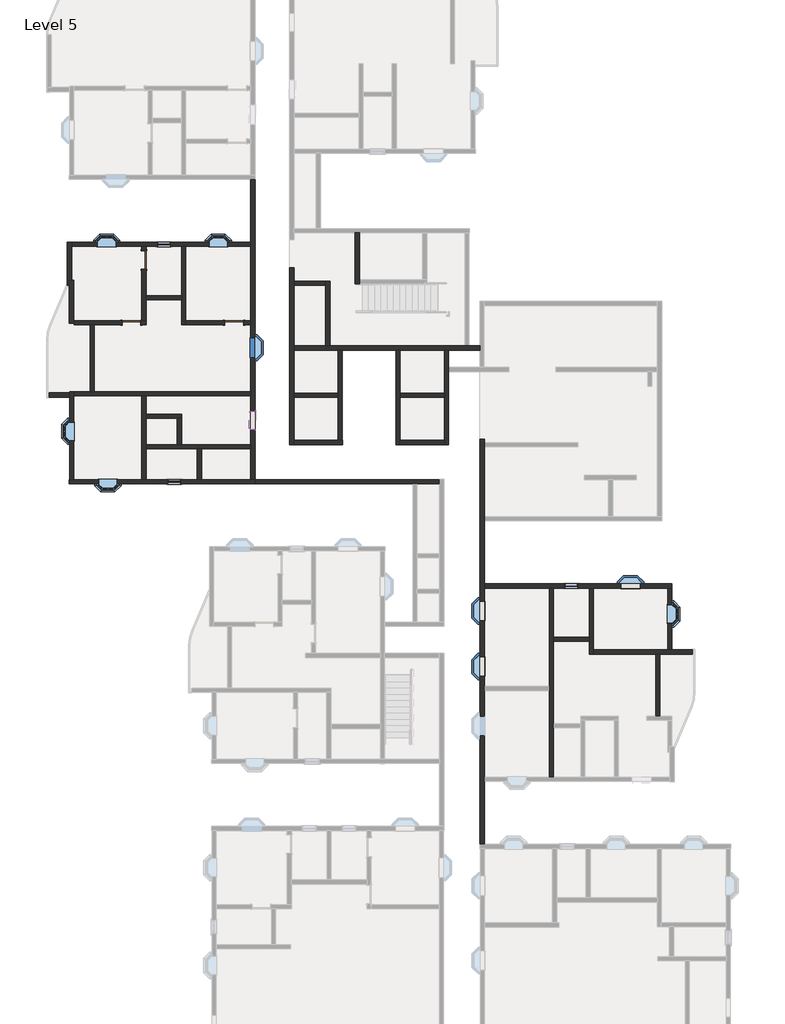
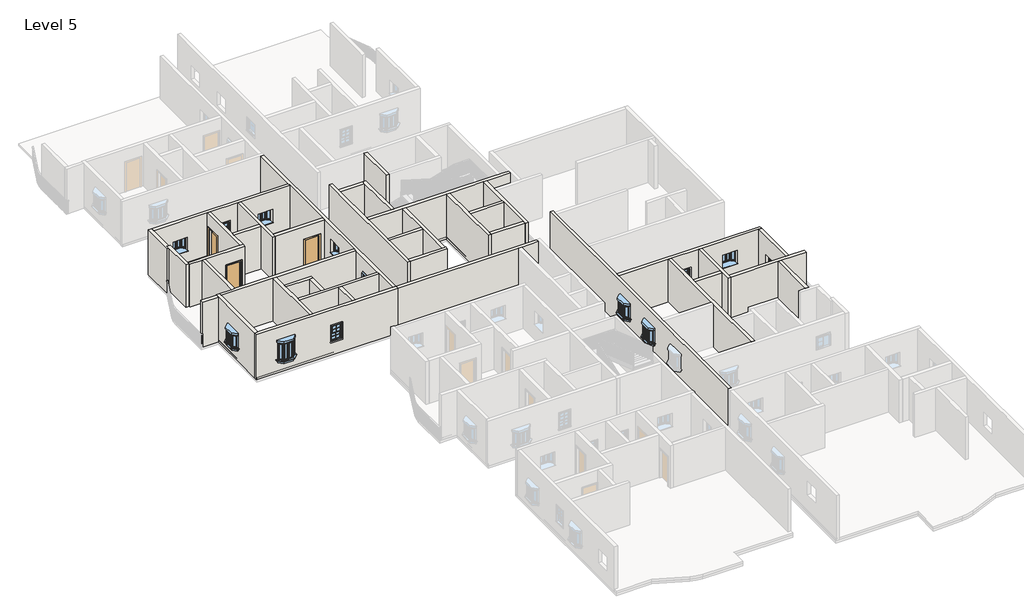
# One storey, part 3 of 14: 40 walls, 13 windows, 3 doors.
"""IFC4 building model written with IfcOpenShell, lengths in millimetres."""

from ifc_helpers import new_model, si_unit, frame, origin, place, context, project, spatial, polyline, outline, extrude, faceted_brep, transform, mapped, element, save
from components import door_54dd4da4, window_910x1210mm_154f9356, window_910x910mm_67ef725a, window_8debb0fa, windows_sgl_w_glazing_bars_910x910mm_256712d0

model = new_model("IFC4")

# Units and contexts
model_context = context("Model", 3, world=origin())
ifc_project = project(units=[si_unit("LENGTHUNIT", "METRE", prefix="MILLI")], contexts=[model_context])

# Site, building, storey
site = spatial("IfcSite", under=ifc_project)
building = spatial("IfcBuilding", under=site)
storey = spatial("IfcBuildingStorey", under=building, Name="Level 5", Elevation=12192.0)

# Doors
placement = place(None, origin())
door_shape = door_54dd4da4(model_context)
element("IfcDoor", 1, ObjectType="Single-Flush : 36\" x 84\"", at=placement, inside=storey, context=model_context, shape_type="MappedRepresentation", body=[
    mapped(door_shape, transform((-11210.3891351, 10605.7083494, 12192.0), x_axis=(1.0, 0.0, 0.0), y_axis=(0.0, 1.0, 0.0), z_axis=(0.0, 0.0, 1.0))),
])
element("IfcDoor", 2, ObjectType="Single-Flush : 36\" x 84\"", at=placement, inside=storey, context=model_context, shape_type="MappedRepresentation", body=[
    mapped(door_shape, transform((-15610.9391351, 13672.7583494, 12192.0), x_axis=(0.0, -1.0, 0.0), y_axis=(1.0, 0.0, 0.0), z_axis=(0.0, 0.0, 1.0))),
])
element("IfcDoor", 3, ObjectType="Single-Flush : 36\" x 84\"", at=placement, inside=storey, context=model_context, shape_type="MappedRepresentation", body=[
    mapped(door_shape, transform((-16220.5391351, 10605.7083494, 12192.0), x_axis=(1.0, 0.0, 0.0), y_axis=(0.0, 1.0, 0.0), z_axis=(0.0, 0.0, 1.0))),
])

# Walls
element("IfcWall", 4, ObjectType="4.5\" p", at=placement, inside=storey, context=model_context, shape_type="Brep", body=[
    faceted_brep([(-15509.3391351, 4456.3873146, 12192.0), (-13007.4391351, 4456.3873146, 12192.0), (-12804.2391351, 4456.3873146, 12192.0), (-10397.5891351, 4456.3873146, 12192.0), (-10397.5891351, 4456.3873146, 15240.0), (-12804.2391351, 4456.3873146, 15240.0), (-13007.4391351, 4456.3873146, 15240.0), (-15509.3391351, 4456.3873146, 15240.0), (-15509.3391351, 4659.5873146, 12192.0), (-15509.3391351, 4659.5873146, 15240.0), (-13985.3391351, 4659.5873146, 15240.0), (-13782.1391351, 4659.5873146, 15240.0), (-10397.5891351, 4659.5873146, 15240.0), (-10397.5891351, 4659.5873146, 12192.0), (-13782.1391351, 4659.5873146, 12192.0), (-13985.3391351, 4659.5873146, 12192.0)], [[[0, 1, 2, 3, 4, 5, 6, 7]], [[8, 9, 10, 11, 12, 13, 14, 15]], [[3, 2, 1, 0, 8, 15, 14, 13]], [[7, 6, 5, 4, 12, 11, 10, 9]], [[4, 3, 13, 12]], [[0, 7, 9, 8]]]),
])
element("IfcWall", 5, ObjectType="4.5\" p", at=placement, inside=storey, context=model_context, shape_type="SweptSolid", body=[
    extrude(outline(polyline([(-13007.4391351, 2953.9583494), (-13007.4391351, 4456.3873146), (-12804.2391351, 4456.3873146), (-12804.2391351, 2953.9583494), (-13007.4391351, 2953.9583494)])), frame((0.0, 0.0, 12192.0), z_axis=(0.0, 0.0, 1.0), x_axis=(1.0, 0.0, 0.0)), (0.0, 0.0, 1.0), 3048.0),
])
element("IfcWall", 6, ObjectType="4.5\" p", at=placement, inside=storey, context=model_context, shape_type="Brep", body=[
    faceted_brep([(-15509.3391351, 5953.2975261, 12192.0), (-13985.3391351, 5953.2975261, 12192.0), (-13782.1391351, 5953.2975261, 12192.0), (-13782.1391351, 5953.2975261, 15240.0), (-13985.3391351, 5953.2975261, 15240.0), (-15509.3391351, 5953.2975261, 15240.0), (-15509.3391351, 6156.4975261, 12192.0), (-15509.3391351, 6156.4975261, 15240.0), (-13782.1391351, 6156.4975261, 15240.0), (-13782.1391351, 6156.4975261, 12192.0)], [[[0, 1, 2, 3, 4, 5]], [[6, 7, 8, 9]], [[2, 1, 0, 6, 9]], [[5, 4, 3, 8, 7]], [[0, 5, 7, 6]], [[3, 2, 9, 8]]]),
])
element("IfcWall", 7, ObjectType="4.5\" p", at=placement, inside=storey, context=model_context, shape_type="SweptSolid", body=[
    extrude(outline(polyline([(-13985.3391351, 4659.5873146), (-13985.3391351, 5953.2975261), (-13782.1391351, 5953.2975261), (-13782.1391351, 4659.5873146), (-13985.3391351, 4659.5873146)])), frame((0.0, 0.0, 12192.0), z_axis=(0.0, 0.0, 1.0), x_axis=(1.0, 0.0, 0.0)), (0.0, 0.0, 1.0), 3048.0),
])
element("IfcWall", 8, ObjectType="4.5\" p", at=placement, inside=storey, context=model_context, shape_type="Brep", body=[
    faceted_brep([(-15712.5391351, 13215.5583494, 14325.6), (-15712.5391351, 13215.5583494, 12192.0), (-15712.5391351, 10707.3083494, 12192.0), (-15712.5391351, 10707.3083494, 15240.0), (-15712.5391351, 14333.1583494, 15240.0), (-15712.5391351, 14333.1583494, 12192.0), (-15712.5391351, 14129.9583494, 12192.0), (-15712.5391351, 14129.9583494, 14325.6), (-15509.3391351, 10707.3083494, 12192.0), (-15509.3391351, 11723.3083494, 12192.0), (-15509.3391351, 11926.5083494, 12192.0), (-15509.3391351, 13215.5583494, 12192.0), (-15509.3391351, 13215.5583494, 14325.6), (-15509.3391351, 14129.9583494, 14325.6), (-15509.3391351, 14129.9583494, 12192.0), (-15509.3391351, 14333.1583494, 12192.0), (-15509.3391351, 14333.1583494, 15240.0), (-15509.3391351, 11926.5083494, 15240.0), (-15509.3391351, 11723.3083494, 15240.0), (-15509.3391351, 10707.3083494, 15240.0)], [[[0, 1, 2, 3, 4, 5, 6, 7]], [[8, 9, 10, 11, 12, 13, 14, 15, 16, 17, 18, 19]], [[6, 5, 15, 14]], [[2, 1, 11, 10, 9, 8]], [[4, 3, 19, 18, 17, 16]], [[3, 2, 8, 19]], [[5, 4, 16, 15]], [[12, 11, 1, 0]], [[13, 12, 0, 7]], [[14, 13, 7, 6]]]),
])
element("IfcWall", 9, ObjectType="4.5\" p", at=placement, inside=storey, context=model_context, shape_type="Brep", body=[
    faceted_brep([(-13769.4391351, 14333.1583494, 12192.0), (-13769.4391351, 11926.5083494, 12192.0), (-13769.4391351, 11723.3083494, 12192.0), (-13769.4391351, 10504.1083494, 12192.0), (-13769.4391351, 10504.1083494, 15240.0), (-13769.4391351, 11723.3083494, 15240.0), (-13769.4391351, 11926.5083494, 15240.0), (-13769.4391351, 14333.1583494, 15240.0), (-13566.2391351, 14333.1583494, 12192.0), (-13566.2391351, 14333.1583494, 15240.0), (-13566.2391351, 10707.3083494, 15240.0), (-13566.2391351, 10504.1083494, 15240.0), (-13566.2391351, 10504.1083494, 12192.0), (-13566.2391351, 10707.3083494, 12192.0)], [[[0, 1, 2, 3, 4, 5, 6, 7]], [[8, 9, 10, 11, 12, 13]], [[3, 2, 1, 0, 8, 13, 12]], [[7, 6, 5, 4, 11, 10, 9]], [[0, 7, 9, 8]], [[4, 3, 12, 11]]]),
])
element("IfcWall", 10, ObjectType="4.5\" p", at=placement, inside=storey, context=model_context, shape_type="SweptSolid", body=[
    extrude(outline(polyline([(14325.6, -10753.1891351), (12192.0, -10753.1891351), (12192.0, -10397.5891351), (15240.0, -10397.5891351), (15240.0, -13566.2391351), (12192.0, -13566.2391351), (12192.0, -11667.5891351), (14325.6, -11667.5891351), (14325.6, -10753.1891351)])), frame((0.0, 10504.1083494, 0.0), z_axis=(0.0, 1.0, 0.0), x_axis=(0.0, 0.0, 1.0)), (0.0, 0.0, 1.0), 203.2),
])
element("IfcWall", 11, ObjectType="4.5\" p", at=placement, inside=storey, context=model_context, shape_type="SweptSolid", body=[
    extrude(outline(polyline([(-13769.4391351, 11723.3083494), (-15509.3391351, 11723.3083494), (-15509.3391351, 11926.5083494), (-13769.4391351, 11926.5083494), (-13769.4391351, 11723.3083494)])), frame((0.0, 0.0, 12192.0), z_axis=(0.0, 0.0, 1.0), x_axis=(1.0, 0.0, 0.0)), (0.0, 0.0, 1.0), 3048.0),
])
element("IfcWall", 12, ObjectType="4.5\" p", at=placement, inside=storey, context=model_context, shape_type="SweptSolid", body=[
    extrude(outline(polyline([(-6739.9891351, 12429.8715905), (-8289.3891351, 12429.8715905), (-8289.3891351, 12633.0715905), (-6739.9891351, 12633.0715905), (-6739.9891351, 12429.8715905)])), frame((0.0, 0.0, 12192.0), z_axis=(0.0, 0.0, 1.0), x_axis=(1.0, 0.0, 0.0)), (0.0, 0.0, 1.0), 3048.0),
])
element("IfcWall", 13, ObjectType="4.5\" p", at=placement, inside=storey, context=model_context, shape_type="SweptSolid", body=[
    extrude(outline(polyline([(-6130.3891351, 6970.2449943), (-8289.3891351, 6970.2449943), (-8289.3891351, 7173.4449943), (-6130.3891351, 7173.4449943), (-6130.3891351, 6970.2449943)])), frame((0.0, 0.0, 12192.0), z_axis=(0.0, 0.0, 1.0), x_axis=(1.0, 0.0, 0.0)), (0.0, 0.0, 1.0), 3048.0),
])
element("IfcWall", 14, ObjectType="4.5\" p", at=placement, inside=storey, context=model_context, shape_type="SweptSolid", body=[
    extrude(outline(polyline([(-948.7891351, 6970.2449943), (-3107.7891351, 6970.2449943), (-3107.7891351, 7173.4449943), (-948.7891351, 7173.4449943), (-948.7891351, 6970.2449943)])), frame((0.0, 0.0, 12192.0), z_axis=(0.0, 0.0, 1.0), x_axis=(1.0, 0.0, 0.0)), (0.0, 0.0, 1.0), 3048.0),
])
element("IfcWall", 15, ObjectType="4.5\" p", at=placement, inside=storey, context=model_context, shape_type="Brep", body=[
    faceted_brep([(-5298.5391351, 14988.9215905, 12192.0), (-5298.5391351, 12506.0715905, 12192.0), (-5298.5391351, 12506.0715905, 15240.0), (-5298.5391351, 14988.9215905, 15240.0), (-5095.3391351, 14988.9215905, 12192.0), (-5095.3391351, 14988.9215905, 15240.0), (-5095.3391351, 12709.2715905, 15240.0), (-5095.3391351, 12506.0715905, 15240.0), (-5095.3391351, 12506.0715905, 12192.0), (-5095.3391351, 12709.2715905, 12192.0)], [[[0, 1, 2, 3]], [[4, 5, 6, 7, 8, 9]], [[1, 0, 4, 9, 8]], [[3, 2, 7, 6, 5]], [[0, 3, 5, 4]], [[2, 1, 8, 7]]]),
])
element("IfcWall", 16, ObjectType="4.5\" p", at=placement, inside=storey, context=model_context, shape_type="SweptSolid", body=[
    extrude(outline(polyline([(-948.7891351, 4665.1949943), (-3107.7891351, 4665.1949943), (-3107.7891351, 4868.3949943), (-948.7891351, 4868.3949943), (-948.7891351, 4665.1949943)])), frame((0.0, 0.0, 12192.0), z_axis=(0.0, 0.0, 1.0), x_axis=(1.0, 0.0, 0.0)), (0.0, 0.0, 1.0), 3048.0),
])
element("IfcWall", 17, ObjectType="4.5\" p", at=placement, inside=storey, context=model_context, shape_type="Brep", body=[
    faceted_brep([(4184.4880523, -2336.4042694, 12192.0), (4184.4880523, -7130.6542694, 12192.0), (4184.4880523, -7333.8542694, 12192.0), (4184.4880523, -11556.6042694, 12192.0), (4184.4880523, -11556.6042694, 15240.0), (4184.4880523, -7333.8542694, 15240.0), (4184.4880523, -7130.6542694, 15240.0), (4184.4880523, -2336.4042694, 15240.0), (4387.6880523, -2336.4042694, 12192.0), (4387.6880523, -2336.4042694, 15240.0), (4387.6880523, -4736.7042694, 15240.0), (4387.6880523, -4939.9042694, 15240.0), (4387.6880523, -8959.4542694, 15240.0), (4387.6880523, -9162.6542694, 15240.0), (4387.6880523, -11556.6042694, 15240.0), (4387.6880523, -11556.6042694, 12192.0), (4387.6880523, -9162.6542694, 12192.0), (4387.6880523, -8959.4542694, 12192.0), (4387.6880523, -4939.9042694, 12192.0), (4387.6880523, -4736.7042694, 12192.0)], [[[0, 1, 2, 3, 4, 5, 6, 7]], [[8, 9, 10, 11, 12, 13, 14, 15, 16, 17, 18, 19]], [[3, 2, 1, 0, 8, 19, 18, 17, 16, 15]], [[7, 6, 5, 4, 14, 13, 12, 11, 10, 9]], [[4, 3, 15, 14]], [[0, 7, 9, 8]]]),
])
element("IfcWall", 18, ObjectType="4.5\" p", at=placement, inside=storey, context=model_context, shape_type="Brep", body=[
    faceted_brep([(803.8108649, 4915.2957306, 12192.0), (803.8108649, -14845.9042694, 12192.0), (803.8108649, -14845.9042694, 15240.0), (803.8108649, 4915.2957306, 15240.0), (803.8108649, -9516.0542694, 14302.0), (803.8108649, -9516.0542694, 13392.0), (803.8108649, -8606.0542694, 13392.0), (803.8108649, -8606.0542694, 14302.0), (803.8108649, -3909.0042694, 14302.0), (803.8108649, -3909.0042694, 13392.0), (803.8108649, -2999.0042694, 13392.0), (803.8108649, -2999.0042694, 14302.0), (803.8108649, -6620.4542694, 14302.0), (803.8108649, -6620.4542694, 13392.0), (803.8108649, -5710.4542694, 13392.0), (803.8108649, -5710.4542694, 14302.0), (1007.0108649, 4915.2957306, 12192.0), (1007.0108649, 4915.2957306, 15240.0), (1007.0108649, 4754.0949943, 15240.0), (1007.0108649, 4550.8949943, 15240.0), (1007.0108649, 1143.3957306, 15240.0), (1007.0108649, 940.1957306, 15240.0), (1007.0108649, -2133.2042694, 15240.0), (1007.0108649, -2336.4042694, 15240.0), (1007.0108649, -7130.6542694, 15240.0), (1007.0108649, -7333.8542694, 15240.0), (1007.0108649, -11556.6042694, 15240.0), (1007.0108649, -11759.8042694, 15240.0), (1007.0108649, -14845.9042694, 15240.0), (1007.0108649, -14845.9042694, 12192.0), (1007.0108649, -11759.8042694, 12192.0), (1007.0108649, -11556.6042694, 12192.0), (1007.0108649, -7333.8542694, 12192.0), (1007.0108649, -7130.6542694, 12192.0), (1007.0108649, -2336.4042694, 12192.0), (1007.0108649, -2133.2042694, 12192.0), (1007.0108649, 940.1957306, 12192.0), (1007.0108649, 1143.3957306, 12192.0), (1007.0108649, 4550.8949943, 12192.0), (1007.0108649, 4754.0949943, 12192.0), (1007.0108649, -9516.0542694, 14302.0), (1007.0108649, -8606.0542694, 14302.0), (1007.0108649, -8606.0542694, 13392.0), (1007.0108649, -9516.0542694, 13392.0), (1007.0108649, -3909.0042694, 14302.0), (1007.0108649, -2999.0042694, 14302.0), (1007.0108649, -2999.0042694, 13392.0), (1007.0108649, -3909.0042694, 13392.0), (1007.0108649, -6620.4542694, 14302.0), (1007.0108649, -5710.4542694, 14302.0), (1007.0108649, -5710.4542694, 13392.0), (1007.0108649, -6620.4542694, 13392.0)], [[[0, 1, 2, 3], [4, 5, 6, 7], [8, 9, 10, 11], [12, 13, 14, 15]], [[16, 17, 18, 19, 20, 21, 22, 23, 24, 25, 26, 27, 28, 29, 30, 31, 32, 33, 34, 35, 36, 37, 38, 39], [40, 41, 42, 43], [44, 45, 46, 47], [48, 49, 50, 51]], [[1, 0, 16, 39, 38, 37, 36, 35, 34, 33, 32, 31, 30, 29]], [[3, 2, 28, 27, 26, 25, 24, 23, 22, 21, 20, 19, 18, 17]], [[0, 3, 17, 16]], [[2, 1, 29, 28]], [[5, 4, 40, 43]], [[6, 5, 43, 42]], [[7, 6, 42, 41]], [[4, 7, 41, 40]], [[9, 8, 44, 47]], [[10, 9, 47, 46]], [[11, 10, 46, 45]], [[8, 11, 45, 44]], [[13, 12, 48, 51]], [[14, 13, 51, 50]], [[15, 14, 50, 49]], [[12, 15, 49, 48]]]),
])
element("IfcWall", 19, ObjectType="4.5\" p", at=placement, inside=storey, context=model_context, shape_type="SweptSolid", body=[
    extrude(outline(polyline([(6127.5880523, -4939.9042694), (4387.6880523, -4939.9042694), (4387.6880523, -4736.7042694), (6127.5880523, -4736.7042694), (6127.5880523, -4939.9042694)])), frame((0.0, 0.0, 12192.0), z_axis=(0.0, 0.0, 1.0), x_axis=(1.0, 0.0, 0.0)), (0.0, 0.0, 1.0), 3048.0),
])
element("IfcWall", 20, ObjectType="4.5\" p", at=placement, inside=storey, context=model_context, shape_type="Brep", body=[
    faceted_brep([(6127.5880523, -2336.4042694, 12192.0), (6127.5880523, -4736.7042694, 12192.0), (6127.5880523, -4939.9042694, 12192.0), (6127.5880523, -5555.8542694, 12192.0), (6127.5880523, -5555.8542694, 15240.0), (6127.5880523, -4939.9042694, 15240.0), (6127.5880523, -4736.7042694, 15240.0), (6127.5880523, -2336.4042694, 15240.0), (6330.7880523, -2336.4042694, 12192.0), (6330.7880523, -2336.4042694, 15240.0), (6330.7880523, -5352.6542694, 15240.0), (6330.7880523, -5555.8542694, 15240.0), (6330.7880523, -5555.8542694, 12192.0), (6330.7880523, -5352.6542694, 12192.0)], [[[0, 1, 2, 3, 4, 5, 6, 7]], [[8, 9, 10, 11, 12, 13]], [[3, 2, 1, 0, 8, 13, 12]], [[7, 6, 5, 4, 11, 10, 9]], [[0, 7, 9, 8]], [[4, 3, 12, 11]]]),
])
element("IfcWall", 21, ObjectType="4.5\" p", at=placement, inside=storey, context=model_context, shape_type="Brep", body=[
    faceted_brep([(6330.7880523, -5555.8542694, 12192.0), (9371.2322031, -5555.8542694, 12192.0), (9574.4322031, -5555.8542694, 12192.0), (11163.1380523, -5555.8542694, 12192.0), (11163.1380523, -5555.8542694, 15240.0), (9574.4322031, -5555.8542694, 15240.0), (9371.2322031, -5555.8542694, 15240.0), (6330.7880523, -5555.8542694, 15240.0), (6330.7880523, -5352.6542694, 12192.0), (6330.7880523, -5352.6542694, 15240.0), (9956.6380523, -5352.6542694, 15240.0), (10159.8380523, -5352.6542694, 15240.0), (11163.1380523, -5352.6542694, 15240.0), (11163.1380523, -5352.6542694, 12192.0), (10159.8380523, -5352.6542694, 12192.0), (9956.6380523, -5352.6542694, 12192.0)], [[[0, 1, 2, 3, 4, 5, 6, 7]], [[8, 9, 10, 11, 12, 13, 14, 15]], [[3, 2, 1, 0, 8, 15, 14, 13]], [[4, 3, 13, 12]], [[7, 6, 5, 4, 12, 11, 10, 9]], [[0, 7, 9, 8]]]),
])
element("IfcWall", 22, ObjectType="4.5\" p", at=placement, inside=storey, context=model_context, shape_type="SweptSolid", body=[
    extrude(outline(polyline([(9371.2322031, -8578.4542694), (9371.2322031, -5555.8542694), (9574.4322031, -5555.8542694), (9574.4322031, -8578.4542694), (9371.2322031, -8578.4542694)])), frame((0.0, 0.0, 12192.0), z_axis=(0.0, 0.0, 1.0), x_axis=(1.0, 0.0, 0.0)), (0.0, 0.0, 1.0), 3048.0),
])
element("IfcWall", 23, ObjectType="9\"", at=placement, inside=storey, context=model_context, shape_type="Brep", body=[
    faceted_brep([(-10181.6891351, 2953.9583494, 12192.0), (-10194.3891351, 2953.9583494, 12192.0), (-10397.5891351, 2953.9583494, 12192.0), (-12804.2391351, 2953.9583494, 12192.0), (-13007.4391351, 2953.9583494, 12192.0), (-15509.3391351, 2953.9583494, 12192.0), (-15712.5391351, 2953.9583494, 12192.0), (-19033.5891351, 2953.9583494, 12192.0), (-19236.7891351, 2953.9583494, 12192.0), (-19249.4891351, 2953.9583494, 12192.0), (-19249.4891351, 2953.9583494, 15240.0), (-19236.7891351, 2953.9583494, 15240.0), (-19033.5891351, 2953.9583494, 15240.0), (-15712.5391351, 2953.9583494, 15240.0), (-15509.3391351, 2953.9583494, 15240.0), (-13007.4391351, 2953.9583494, 15240.0), (-12804.2391351, 2953.9583494, 15240.0), (-10397.5891351, 2953.9583494, 15240.0), (-10194.3891351, 2953.9583494, 15240.0), (-10181.6891351, 2953.9583494, 15240.0), (-13794.8391351, 2953.9583494, 14173.2), (-14455.2391351, 2953.9583494, 14173.2), (-14455.2391351, 2953.9583494, 13106.4), (-13794.8391351, 2953.9583494, 13106.4), (-16918.0641351, 2953.9583494, 14302.0), (-17828.0641351, 2953.9583494, 14302.0), (-17828.0641351, 2953.9583494, 13092.0), (-16918.0641351, 2953.9583494, 13092.0), (-10181.6891351, 2750.7583494, 12192.0), (-10181.6891351, 2750.7583494, 15240.0), (-19249.4891351, 2750.7583494, 15240.0), (-19249.4891351, 2750.7583494, 12192.0), (-13794.8391351, 2750.7583494, 14173.2), (-13794.8391351, 2750.7583494, 13106.4), (-14455.2391351, 2750.7583494, 13106.4), (-14455.2391351, 2750.7583494, 14173.2), (-16918.0641351, 2750.7583494, 14302.0), (-16918.0641351, 2750.7583494, 13092.0), (-17828.0641351, 2750.7583494, 13092.0), (-17828.0641351, 2750.7583494, 14302.0)], [[[0, 1, 2, 3, 4, 5, 6, 7, 8, 9, 10, 11, 12, 13, 14, 15, 16, 17, 18, 19], [20, 21, 22, 23], [24, 25, 26, 27]], [[28, 29, 30, 31], [32, 33, 34, 35], [36, 37, 38, 39]], [[9, 8, 7, 6, 5, 4, 3, 2, 1, 0, 28, 31]], [[10, 9, 31, 30]], [[19, 18, 17, 16, 15, 14, 13, 12, 11, 10, 30, 29]], [[0, 19, 29, 28]], [[33, 32, 20, 23]], [[34, 33, 23, 22]], [[35, 34, 22, 21]], [[32, 35, 21, 20]], [[37, 36, 24, 27]], [[38, 37, 27, 26]], [[39, 38, 26, 25]], [[36, 39, 25, 24]]]),
])
element("IfcWall", 24, ObjectType="9\"", at=placement, inside=storey, context=model_context, shape_type="Brep", body=[
    faceted_brep([(-19033.5891351, 2953.9583494, 12192.0), (-19033.5891351, 7037.0083494, 12192.0), (-19033.5891351, 7240.2083494, 12192.0), (-19033.5891351, 7240.2083494, 15240.0), (-19033.5891351, 7037.0083494, 15240.0), (-19033.5891351, 2953.9583494, 15240.0), (-19033.5891351, 4854.8083494, 14016.4), (-19033.5891351, 5764.8083494, 14016.4), (-19033.5891351, 5764.8083494, 13106.4), (-19033.5891351, 4854.8083494, 13106.4), (-19236.7891351, 2953.9583494, 12192.0), (-19236.7891351, 2953.9583494, 15240.0), (-19236.7891351, 7240.2083494, 15240.0), (-19236.7891351, 7240.2083494, 12192.0), (-19236.7891351, 4854.8083494, 14016.4), (-19236.7891351, 4854.8083494, 13106.4), (-19236.7891351, 5764.8083494, 13106.4), (-19236.7891351, 5764.8083494, 14016.4)], [[[0, 1, 2, 3, 4, 5], [6, 7, 8, 9]], [[10, 11, 12, 13], [14, 15, 16, 17]], [[2, 1, 0, 10, 13]], [[5, 4, 3, 12, 11]], [[0, 5, 11, 10]], [[3, 2, 13, 12]], [[15, 14, 6, 9]], [[16, 15, 9, 8]], [[17, 16, 8, 7]], [[14, 17, 7, 6]]]),
])
element("IfcWall", 25, ObjectType="9\"", at=placement, inside=storey, context=model_context, shape_type="Brep", body=[
    faceted_brep([(-10194.3891351, 2953.9583494, 12192.0), (-10194.3891351, 17597.0583494, 12192.0), (-10194.3891351, 17597.0583494, 15240.0), (-10194.3891351, 2953.9583494, 15240.0), (-10194.3891351, 9841.5083494, 14302.0), (-10194.3891351, 9841.5083494, 13392.0), (-10194.3891351, 8931.5083494, 13392.0), (-10194.3891351, 8931.5083494, 14302.0), (-10194.3891351, 5393.297832, 14302.0), (-10194.3891351, 6303.297832, 14302.0), (-10194.3891351, 6303.297832, 13392.0), (-10194.3891351, 5393.297832, 13392.0), (-10397.5891351, 2953.9583494, 12192.0), (-10397.5891351, 2953.9583494, 15240.0), (-10397.5891351, 4456.3873146, 15240.0), (-10397.5891351, 4659.5873146, 15240.0), (-10397.5891351, 7037.0083494, 15240.0), (-10397.5891351, 7240.2083494, 15240.0), (-10397.5891351, 10504.1083494, 15240.0), (-10397.5891351, 10707.3083494, 15240.0), (-10397.5891351, 14333.1583494, 15240.0), (-10397.5891351, 14536.3583494, 15240.0), (-10397.5891351, 17597.0583494, 15240.0), (-10397.5891351, 17597.0583494, 12192.0), (-10397.5891351, 14536.3583494, 12192.0), (-10397.5891351, 14333.1583494, 12192.0), (-10397.5891351, 10707.3083494, 12192.0), (-10397.5891351, 10504.1083494, 12192.0), (-10397.5891351, 7240.2083494, 12192.0), (-10397.5891351, 7037.0083494, 12192.0), (-10397.5891351, 4659.5873146, 12192.0), (-10397.5891351, 4456.3873146, 12192.0), (-10397.5891351, 9841.5083494, 14302.0), (-10397.5891351, 8931.5083494, 14302.0), (-10397.5891351, 8931.5083494, 13392.0), (-10397.5891351, 9841.5083494, 13392.0), (-10397.5891351, 5393.297832, 14302.0), (-10397.5891351, 5393.297832, 13392.0), (-10397.5891351, 6303.297832, 13392.0), (-10397.5891351, 6303.297832, 14302.0)], [[[0, 1, 2, 3], [4, 5, 6, 7], [8, 9, 10, 11]], [[12, 13, 14, 15, 16, 17, 18, 19, 20, 21, 22, 23, 24, 25, 26, 27, 28, 29, 30, 31], [32, 33, 34, 35], [36, 37, 38, 39]], [[1, 0, 12, 31, 30, 29, 28, 27, 26, 25, 24, 23]], [[2, 1, 23, 22]], [[3, 2, 22, 21, 20, 19, 18, 17, 16, 15, 14, 13]], [[0, 3, 13, 12]], [[5, 4, 32, 35]], [[6, 5, 35, 34]], [[7, 6, 34, 33]], [[4, 7, 33, 32]], [[37, 36, 8, 11]], [[38, 37, 11, 10]], [[39, 38, 10, 9]], [[36, 39, 9, 8]]]),
])
element("IfcWall", 26, ObjectType="9\"", at=placement, inside=storey, context=model_context, shape_type="SweptSolid", body=[
    extrude(outline(polyline([(-19249.4891351, 6979.8583494), (-20240.0891351, 6979.8583494), (-20240.0891351, 7183.0583494), (-19249.4891351, 7183.0583494), (-19249.4891351, 6979.8583494)])), frame((0.0, 0.0, 12192.0), z_axis=(0.0, 0.0, 1.0), x_axis=(1.0, 0.0, 0.0)), (0.0, 0.0, 1.0), 3048.0),
])
element("IfcWall", 27, ObjectType="9\"", at=placement, inside=storey, context=model_context, shape_type="Brep", body=[
    faceted_brep([(-19147.8891351, 12435.1858981, 12192.0), (-19147.8891351, 14333.1583494, 12192.0), (-19147.8891351, 14536.3583494, 12192.0), (-19147.8891351, 14549.0583494, 12192.0), (-19147.8891351, 14549.0583494, 15240.0), (-19147.8891351, 14536.3583494, 15240.0), (-19147.8891351, 14333.1583494, 15240.0), (-19147.8891351, 12435.1858981, 15240.0), (-19351.0891351, 12435.1858981, 12192.0), (-19351.0891351, 12435.1858981, 15240.0), (-19351.0891351, 14549.0583494, 15240.0), (-19351.0891351, 14549.0583494, 12192.0)], [[[0, 1, 2, 3, 4, 5, 6, 7]], [[8, 9, 10, 11]], [[3, 2, 1, 0, 8, 11]], [[4, 3, 11, 10]], [[7, 6, 5, 4, 10, 9]], [[0, 7, 9, 8]]]),
])
element("IfcWall", 28, ObjectType="9\"", at=placement, inside=storey, context=model_context, shape_type="Brep", body=[
    faceted_brep([(-19147.8891351, 14333.1583494, 12192.0), (-15712.5391351, 14333.1583494, 12192.0), (-15509.3391351, 14333.1583494, 12192.0), (-13769.4391351, 14333.1583494, 12192.0), (-13566.2391351, 14333.1583494, 12192.0), (-10397.5891351, 14333.1583494, 12192.0), (-10397.5891351, 14333.1583494, 15240.0), (-13566.2391351, 14333.1583494, 15240.0), (-13769.4391351, 14333.1583494, 15240.0), (-15509.3391351, 14333.1583494, 15240.0), (-15712.5391351, 14333.1583494, 15240.0), (-19147.8891351, 14333.1583494, 15240.0), (-17885.2141351, 14333.1583494, 14016.4), (-16975.2141351, 14333.1583494, 14016.4), (-16975.2141351, 14333.1583494, 13106.4), (-17885.2141351, 14333.1583494, 13106.4), (-12436.9141351, 14333.1583494, 14016.4), (-11526.9141351, 14333.1583494, 14016.4), (-11526.9141351, 14333.1583494, 13106.4), (-12436.9141351, 14333.1583494, 13106.4), (-14309.1891351, 14333.1583494, 14173.2), (-14309.1891351, 14333.1583494, 13106.4), (-14969.5891351, 14333.1583494, 13106.4), (-14969.5891351, 14333.1583494, 14173.2), (-19147.8891351, 14536.3583494, 12192.0), (-19147.8891351, 14536.3583494, 15240.0), (-10397.5891351, 14536.3583494, 15240.0), (-10397.5891351, 14536.3583494, 12192.0), (-17885.2141351, 14536.3583494, 14016.4), (-17885.2141351, 14536.3583494, 13106.4), (-16975.2141351, 14536.3583494, 13106.4), (-16975.2141351, 14536.3583494, 14016.4), (-12436.9141351, 14536.3583494, 14016.4), (-12436.9141351, 14536.3583494, 13106.4), (-11526.9141351, 14536.3583494, 13106.4), (-11526.9141351, 14536.3583494, 14016.4), (-14309.1891351, 14536.3583494, 14173.2), (-14969.5891351, 14536.3583494, 14173.2), (-14969.5891351, 14536.3583494, 13106.4), (-14309.1891351, 14536.3583494, 13106.4)], [[[0, 1, 2, 3, 4, 5, 6, 7, 8, 9, 10, 11], [12, 13, 14, 15], [16, 17, 18, 19], [20, 21, 22, 23]], [[24, 25, 26, 27], [28, 29, 30, 31], [32, 33, 34, 35], [36, 37, 38, 39]], [[5, 4, 3, 2, 1, 0, 24, 27]], [[11, 10, 9, 8, 7, 6, 26, 25]], [[6, 5, 27, 26]], [[0, 11, 25, 24]], [[29, 28, 12, 15]], [[30, 29, 15, 14]], [[31, 30, 14, 13]], [[28, 31, 13, 12]], [[33, 32, 16, 19]], [[34, 33, 19, 18]], [[35, 34, 18, 17]], [[32, 35, 17, 16]], [[21, 20, 36, 39]], [[22, 21, 39, 38]], [[23, 22, 38, 37]], [[20, 23, 37, 36]]]),
])
element("IfcWall", 29, ObjectType="9\"", at=placement, inside=storey, context=model_context, shape_type="SweptSolid", body=[
    extrude(outline(polyline([(-19249.4891351, 10585.5474528), (-19249.4891351, 12672.4473407), (-19046.2891351, 12672.4473407), (-19046.2891351, 10585.5474528), (-19249.4891351, 10585.5474528)])), frame((0.0, 0.0, 12192.0), z_axis=(0.0, 0.0, 1.0), x_axis=(1.0, 0.0, 0.0)), (0.0, 0.0, 1.0), 3048.0),
])
element("IfcWall", 30, ObjectType="9\" w", at=placement, inside=storey, context=model_context, shape_type="Brep", body=[
    faceted_brep([(-1177.3891351, 2953.9583494, 12192.0), (-10181.6891351, 2953.9583494, 12192.0), (-10181.6891351, 2953.9583494, 15240.0), (-1177.3891351, 2953.9583494, 15240.0), (-1177.3891351, 2750.7583494, 12192.0), (-1177.3891351, 2750.7583494, 15240.0), (-2269.5891351, 2750.7583494, 15240.0), (-2472.7891351, 2750.7583494, 15240.0), (-10181.6891351, 2750.7583494, 15240.0), (-10181.6891351, 2750.7583494, 12192.0), (-2472.7891351, 2750.7583494, 12192.0), (-2269.5891351, 2750.7583494, 12192.0)], [[[0, 1, 2, 3]], [[4, 5, 6, 7, 8, 9, 10, 11]], [[1, 0, 4, 11, 10, 9]], [[2, 1, 9, 8]], [[3, 2, 8, 7, 6, 5]], [[0, 3, 5, 4]]]),
])
element("IfcWall", 31, ObjectType="9\" w", at=placement, inside=storey, context=model_context, shape_type="Brep", body=[
    faceted_brep([(-15763.3391351, 10504.1083494, 14325.6), (-15763.3391351, 10504.1083494, 12192.0), (-15509.3391351, 10504.1083494, 12192.0), (-15509.3391351, 10504.1083494, 15240.0), (-18042.9891351, 10504.1083494, 15240.0), (-18246.1891351, 10504.1083494, 15240.0), (-19027.2391351, 10504.1083494, 15240.0), (-19027.2391351, 10504.1083494, 12192.0), (-18246.1891351, 10504.1083494, 12192.0), (-18042.9891351, 10504.1083494, 12192.0), (-16677.7391351, 10504.1083494, 12192.0), (-16677.7391351, 10504.1083494, 14325.6), (-15509.3391351, 10707.3083494, 12192.0), (-15712.5391351, 10707.3083494, 12192.0), (-15763.3391351, 10707.3083494, 12192.0), (-15763.3391351, 10707.3083494, 14325.6), (-16677.7391351, 10707.3083494, 14325.6), (-16677.7391351, 10707.3083494, 12192.0), (-19027.2391351, 10707.3083494, 12192.0), (-19027.2391351, 10707.3083494, 15240.0), (-15712.5391351, 10707.3083494, 15240.0), (-15509.3391351, 10707.3083494, 15240.0)], [[[0, 1, 2, 3, 4, 5, 6, 7, 8, 9, 10, 11]], [[12, 13, 14, 15, 16, 17, 18, 19, 20, 21]], [[2, 1, 14, 13, 12]], [[10, 9, 8, 7, 18, 17]], [[6, 5, 4, 3, 21, 20, 19]], [[7, 6, 19, 18]], [[3, 2, 12, 21]], [[15, 14, 1, 0]], [[16, 15, 0, 11]], [[17, 16, 11, 10]]]),
])
element("IfcWall", 32, ObjectType="9\" w", at=placement, inside=storey, context=model_context, shape_type="SweptSolid", body=[
    extrude(outline(polyline([(-18246.1891351, 7240.2083494), (-18246.1891351, 10504.1083494), (-18042.9891351, 10504.1083494), (-18042.9891351, 7240.2083494), (-18246.1891351, 7240.2083494)])), frame((0.0, 0.0, 12192.0), z_axis=(0.0, 0.0, 1.0), x_axis=(1.0, 0.0, 0.0)), (0.0, 0.0, 1.0), 3048.0),
])
element("IfcWall", 33, ObjectType="9\" w", at=placement, inside=storey, context=model_context, shape_type="Brep", body=[
    faceted_brep([(-19033.5891351, 7037.0083494, 12192.0), (-15712.5391351, 7037.0083494, 12192.0), (-15509.3391351, 7037.0083494, 12192.0), (-10397.5891351, 7037.0083494, 12192.0), (-10397.5891351, 7037.0083494, 15240.0), (-15509.3391351, 7037.0083494, 15240.0), (-15712.5391351, 7037.0083494, 15240.0), (-19033.5891351, 7037.0083494, 15240.0), (-19033.5891351, 7240.2083494, 12192.0), (-19033.5891351, 7240.2083494, 15240.0), (-18246.1891351, 7240.2083494, 15240.0), (-18042.9891351, 7240.2083494, 15240.0), (-10397.5891351, 7240.2083494, 15240.0), (-10397.5891351, 7240.2083494, 12192.0), (-18042.9891351, 7240.2083494, 12192.0), (-18246.1891351, 7240.2083494, 12192.0)], [[[0, 1, 2, 3, 4, 5, 6, 7]], [[8, 9, 10, 11, 12, 13, 14, 15]], [[3, 2, 1, 0, 8, 15, 14, 13]], [[7, 6, 5, 4, 12, 11, 10, 9]], [[0, 7, 9, 8]], [[4, 3, 13, 12]]]),
])
element("IfcWall", 34, ObjectType="9\" w", at=placement, inside=storey, context=model_context, shape_type="Brep", body=[
    faceted_brep([(-15712.5391351, 7037.0083494, 12192.0), (-15712.5391351, 2953.9583494, 12192.0), (-15712.5391351, 2953.9583494, 15240.0), (-15712.5391351, 7037.0083494, 15240.0), (-15509.3391351, 7037.0083494, 12192.0), (-15509.3391351, 7037.0083494, 15240.0), (-15509.3391351, 6156.4975261, 15240.0), (-15509.3391351, 5953.2975261, 15240.0), (-15509.3391351, 4659.5873146, 15240.0), (-15509.3391351, 4456.3873146, 15240.0), (-15509.3391351, 2953.9583494, 15240.0), (-15509.3391351, 2953.9583494, 12192.0), (-15509.3391351, 4456.3873146, 12192.0), (-15509.3391351, 4659.5873146, 12192.0), (-15509.3391351, 5953.2975261, 12192.0), (-15509.3391351, 6156.4975261, 12192.0)], [[[0, 1, 2, 3]], [[4, 5, 6, 7, 8, 9, 10, 11, 12, 13, 14, 15]], [[1, 0, 4, 15, 14, 13, 12, 11]], [[3, 2, 10, 9, 8, 7, 6, 5]], [[2, 1, 11, 10]], [[0, 3, 5, 4]]]),
])
element("IfcWall", 35, ObjectType="9\" w", at=placement, inside=storey, context=model_context, shape_type="Brep", body=[
    faceted_brep([(-8492.5891351, 13295.1410318, 12192.0), (-8492.5891351, 4652.4949943, 12192.0), (-8492.5891351, 4652.4949943, 15240.0), (-8492.5891351, 13295.1410318, 15240.0), (-8289.3891351, 13295.1410318, 12192.0), (-8289.3891351, 13295.1410318, 15240.0), (-8289.3891351, 12633.0715905, 15240.0), (-8289.3891351, 12429.8715905, 15240.0), (-8289.3891351, 9478.4949943, 15240.0), (-8289.3891351, 9275.2949943, 15240.0), (-8289.3891351, 7173.4449943, 15240.0), (-8289.3891351, 6970.2449943, 15240.0), (-8289.3891351, 4868.3949943, 15240.0), (-8289.3891351, 4665.1949943, 15240.0), (-8289.3891351, 4652.4949943, 15240.0), (-8289.3891351, 4652.4949943, 12192.0), (-8289.3891351, 4665.1949943, 12192.0), (-8289.3891351, 4868.3949943, 12192.0), (-8289.3891351, 6970.2449943, 12192.0), (-8289.3891351, 7173.4449943, 12192.0), (-8289.3891351, 9275.2949943, 12192.0), (-8289.3891351, 9478.4949943, 12192.0), (-8289.3891351, 12429.8715905, 12192.0), (-8289.3891351, 12633.0715905, 12192.0)], [[[0, 1, 2, 3]], [[4, 5, 6, 7, 8, 9, 10, 11, 12, 13, 14, 15, 16, 17, 18, 19, 20, 21, 22, 23]], [[1, 0, 4, 23, 22, 21, 20, 19, 18, 17, 16, 15]], [[2, 1, 15, 14]], [[3, 2, 14, 13, 12, 11, 10, 9, 8, 7, 6, 5]], [[0, 3, 5, 4]]]),
])
element("IfcWall", 36, ObjectType="9\" w", at=placement, inside=storey, context=model_context, shape_type="Brep", body=[
    faceted_brep([(-8289.3891351, 4665.1949943, 12192.0), (-5914.4891351, 4665.1949943, 12192.0), (-5914.4891351, 4665.1949943, 15240.0), (-8289.3891351, 4665.1949943, 15240.0), (-8289.3891351, 4868.3949943, 12192.0), (-8289.3891351, 4868.3949943, 15240.0), (-6130.3891351, 4868.3949943, 15240.0), (-5927.1891351, 4868.3949943, 15240.0), (-5914.4891351, 4868.3949943, 15240.0), (-5914.4891351, 4868.3949943, 12192.0), (-5927.1891351, 4868.3949943, 12192.0), (-6130.3891351, 4868.3949943, 12192.0)], [[[0, 1, 2, 3]], [[4, 5, 6, 7, 8, 9, 10, 11]], [[1, 0, 4, 11, 10, 9]], [[2, 1, 9, 8]], [[3, 2, 8, 7, 6, 5]], [[0, 3, 5, 4]]]),
])
element("IfcWall", 37, ObjectType="9\" w", at=placement, inside=storey, context=model_context, shape_type="Brep", body=[
    faceted_brep([(-5927.1891351, 4868.3949943, 12192.0), (-5927.1891351, 9275.2949943, 12192.0), (-5927.1891351, 9275.2949943, 15240.0), (-5927.1891351, 4868.3949943, 15240.0), (-6130.3891351, 4868.3949943, 12192.0), (-6130.3891351, 4868.3949943, 15240.0), (-6130.3891351, 6970.2449943, 15240.0), (-6130.3891351, 7173.4449943, 15240.0), (-6130.3891351, 9275.2949943, 15240.0), (-6130.3891351, 9275.2949943, 12192.0), (-6130.3891351, 7173.4449943, 12192.0), (-6130.3891351, 6970.2449943, 12192.0)], [[[0, 1, 2, 3]], [[4, 5, 6, 7, 8, 9, 10, 11]], [[1, 0, 4, 11, 10, 9]], [[3, 2, 8, 7, 6, 5]], [[0, 3, 5, 4]], [[2, 1, 9, 8]]]),
])
element("IfcWall", 38, ObjectType="9\" w", at=placement, inside=storey, context=model_context, shape_type="Brep", body=[
    faceted_brep([(-8289.3891351, 9275.2949943, 12192.0), (-6130.3891351, 9275.2949943, 12192.0), (-5927.1891351, 9275.2949943, 12192.0), (-3310.9891351, 9275.2949943, 12192.0), (-3107.7891351, 9275.2949943, 12192.0), (-948.7891351, 9275.2949943, 12192.0), (-745.5891351, 9275.2949943, 12192.0), (793.5880523, 9275.2949943, 12192.0), (793.5880523, 9275.2949943, 15240.0), (-745.5891351, 9275.2949943, 15240.0), (-948.7891351, 9275.2949943, 15240.0), (-3107.7891351, 9275.2949943, 15240.0), (-3310.9891351, 9275.2949943, 15240.0), (-5927.1891351, 9275.2949943, 15240.0), (-6130.3891351, 9275.2949943, 15240.0), (-8289.3891351, 9275.2949943, 15240.0), (-8289.3891351, 9478.4949943, 12192.0), (-8289.3891351, 9478.4949943, 15240.0), (-6739.9891351, 9478.4949943, 15240.0), (-6536.7891351, 9478.4949943, 15240.0), (54.5108649, 9478.4949943, 15240.0), (257.7108649, 9478.4949943, 15240.0), (793.5880523, 9478.4949943, 15240.0), (793.5880523, 9478.4949943, 12192.0), (257.7108649, 9478.4949943, 12192.0), (54.5108649, 9478.4949943, 12192.0), (-6536.7891351, 9478.4949943, 12192.0), (-6739.9891351, 9478.4949943, 12192.0)], [[[0, 1, 2, 3, 4, 5, 6, 7, 8, 9, 10, 11, 12, 13, 14, 15]], [[16, 17, 18, 19, 20, 21, 22, 23, 24, 25, 26, 27]], [[7, 6, 5, 4, 3, 2, 1, 0, 16, 27, 26, 25, 24, 23]], [[15, 14, 13, 12, 11, 10, 9, 8, 22, 21, 20, 19, 18, 17]], [[0, 15, 17, 16]], [[8, 7, 23, 22]]]),
])
element("IfcWall", 39, ObjectType="9\" w", at=placement, inside=storey, context=model_context, shape_type="Brep", body=[
    faceted_brep([(-3310.9891351, 9275.2949943, 12192.0), (-3310.9891351, 4652.4949943, 12192.0), (-3310.9891351, 4652.4949943, 15240.0), (-3310.9891351, 9275.2949943, 15240.0), (-3107.7891351, 9275.2949943, 12192.0), (-3107.7891351, 9275.2949943, 15240.0), (-3107.7891351, 7173.4449943, 15240.0), (-3107.7891351, 6970.2449943, 15240.0), (-3107.7891351, 4868.3949943, 15240.0), (-3107.7891351, 4665.1949943, 15240.0), (-3107.7891351, 4652.4949943, 15240.0), (-3107.7891351, 4652.4949943, 12192.0), (-3107.7891351, 4665.1949943, 12192.0), (-3107.7891351, 4868.3949943, 12192.0), (-3107.7891351, 6970.2449943, 12192.0), (-3107.7891351, 7173.4449943, 12192.0)], [[[0, 1, 2, 3]], [[4, 5, 6, 7, 8, 9, 10, 11, 12, 13, 14, 15]], [[1, 0, 4, 15, 14, 13, 12, 11]], [[2, 1, 11, 10]], [[3, 2, 10, 9, 8, 7, 6, 5]], [[0, 3, 5, 4]]]),
])
element("IfcWall", 40, ObjectType="9\" w", at=placement, inside=storey, context=model_context, shape_type="Brep", body=[
    faceted_brep([(-745.5891351, 4652.4949943, 12192.0), (-745.5891351, 8223.6457306, 12192.0), (-745.5891351, 8426.8457306, 12192.0), (-745.5891351, 9275.2949943, 12192.0), (-745.5891351, 9275.2949943, 15240.0), (-745.5891351, 8426.8457306, 15240.0), (-745.5891351, 8223.6457306, 15240.0), (-745.5891351, 4652.4949943, 15240.0), (-948.7891351, 4652.4949943, 12192.0), (-948.7891351, 4652.4949943, 15240.0), (-948.7891351, 4665.1949943, 15240.0), (-948.7891351, 4868.3949943, 15240.0), (-948.7891351, 6970.2449943, 15240.0), (-948.7891351, 7173.4449943, 15240.0), (-948.7891351, 9275.2949943, 15240.0), (-948.7891351, 9275.2949943, 12192.0), (-948.7891351, 7173.4449943, 12192.0), (-948.7891351, 6970.2449943, 12192.0), (-948.7891351, 4868.3949943, 12192.0), (-948.7891351, 4665.1949943, 12192.0)], [[[0, 1, 2, 3, 4, 5, 6, 7]], [[8, 9, 10, 11, 12, 13, 14, 15, 16, 17, 18, 19]], [[3, 2, 1, 0, 8, 19, 18, 17, 16, 15]], [[7, 6, 5, 4, 14, 13, 12, 11, 10, 9]], [[0, 7, 9, 8]], [[4, 3, 15, 14]]]),
])
element("IfcWall", 41, ObjectType="9\" w", at=placement, inside=storey, context=model_context, shape_type="Brep", body=[
    faceted_brep([(-6536.7891351, 9478.4949943, 12192.0), (-6536.7891351, 12633.0715905, 12192.0), (-6536.7891351, 12633.0715905, 15240.0), (-6536.7891351, 9478.4949943, 15240.0), (-6739.9891351, 9478.4949943, 12192.0), (-6739.9891351, 9478.4949943, 15240.0), (-6739.9891351, 12429.8715905, 15240.0), (-6739.9891351, 12633.0715905, 15240.0), (-6739.9891351, 12633.0715905, 12192.0), (-6739.9891351, 12429.8715905, 12192.0)], [[[0, 1, 2, 3]], [[4, 5, 6, 7, 8, 9]], [[1, 0, 4, 9, 8]], [[3, 2, 7, 6, 5]], [[0, 3, 5, 4]], [[2, 1, 8, 7]]]),
])
element("IfcWall", 42, ObjectType="9\" w", at=placement, inside=storey, context=model_context, shape_type="Brep", body=[
    faceted_brep([(1007.0108649, -2336.4042694, 12192.0), (4184.4880523, -2336.4042694, 12192.0), (4387.6880523, -2336.4042694, 12192.0), (6127.5880523, -2336.4042694, 12192.0), (6330.7880523, -2336.4042694, 12192.0), (9956.6380523, -2336.4042694, 12192.0), (10159.8380523, -2336.4042694, 12192.0), (10172.5380523, -2336.4042694, 12192.0), (10172.5380523, -2336.4042694, 15240.0), (10159.8380523, -2336.4042694, 15240.0), (9956.6380523, -2336.4042694, 15240.0), (6330.7880523, -2336.4042694, 15240.0), (6127.5880523, -2336.4042694, 15240.0), (4387.6880523, -2336.4042694, 15240.0), (4184.4880523, -2336.4042694, 15240.0), (1007.0108649, -2336.4042694, 15240.0), (7688.7130523, -2336.4042694, 14302.0), (8598.7130523, -2336.4042694, 14302.0), (8598.7130523, -2336.4042694, 13392.0), (7688.7130523, -2336.4042694, 13392.0), (4927.4380523, -2336.4042694, 14173.2), (5587.8380523, -2336.4042694, 14173.2), (5587.8380523, -2336.4042694, 13106.4), (4927.4380523, -2336.4042694, 13106.4), (1007.0108649, -2133.2042694, 12192.0), (1007.0108649, -2133.2042694, 15240.0), (10172.5380523, -2133.2042694, 15240.0), (10172.5380523, -2133.2042694, 12192.0), (7688.7130523, -2133.2042694, 14302.0), (7688.7130523, -2133.2042694, 13392.0), (8598.7130523, -2133.2042694, 13392.0), (8598.7130523, -2133.2042694, 14302.0), (4927.4380523, -2133.2042694, 14173.2), (4927.4380523, -2133.2042694, 13106.4), (5587.8380523, -2133.2042694, 13106.4), (5587.8380523, -2133.2042694, 14173.2)], [[[0, 1, 2, 3, 4, 5, 6, 7, 8, 9, 10, 11, 12, 13, 14, 15], [16, 17, 18, 19], [20, 21, 22, 23]], [[24, 25, 26, 27], [28, 29, 30, 31], [32, 33, 34, 35]], [[7, 6, 5, 4, 3, 2, 1, 0, 24, 27]], [[8, 7, 27, 26]], [[15, 14, 13, 12, 11, 10, 9, 8, 26, 25]], [[0, 15, 25, 24]], [[29, 28, 16, 19]], [[30, 29, 19, 18]], [[31, 30, 18, 17]], [[28, 31, 17, 16]], [[33, 32, 20, 23]], [[34, 33, 23, 22]], [[35, 34, 22, 21]], [[32, 35, 21, 20]]]),
])
element("IfcWall", 43, ObjectType="9\" w", at=placement, inside=storey, context=model_context, shape_type="SweptSolid", body=[
    extrude(outline(polyline([(-2336.4042694, 12192.0), (-5352.6542694, 12192.0), (-5352.6542694, 15240.0), (-2336.4042694, 15240.0), (-2336.4042694, 12192.0)]), holes=[polyline([(-3151.4042694, 14016.4), (-4061.4042694, 14016.4), (-4061.4042694, 13106.4), (-3151.4042694, 13106.4), (-3151.4042694, 14016.4)])]), frame((9956.6380523, 0.0, 0.0), z_axis=(1.0, 0.0, 0.0), x_axis=(0.0, 1.0, 0.0)), (0.0, 0.0, 1.0), 203.2),
])

# Windows
window_910x1210mm_shape = window_910x1210mm_154f9356(model_context)
element("IfcWindow", 44, ObjectType="910x1210mm", at=placement, inside=storey, context=model_context, shape_type="MappedRepresentation", body=[
    mapped(window_910x1210mm_shape, transform((-17943.0641351, 2860.8149172, 12192.0), x_axis=(-1.0, 0.0, 0.0), y_axis=(0.0, -1.0, 0.0), z_axis=(0.0, 0.0, 1.0))),
])
window_910x910mm_shape = window_910x910mm_67ef725a(model_context)
element("IfcWindow", 45, ObjectType="910x910mm", at=placement, inside=storey, context=model_context, shape_type="MappedRepresentation", body=[
    mapped(window_910x910mm_shape, transform((8713.7130523, -2243.2608372, 12192.0), x_axis=(1.0, 0.0, 0.0), y_axis=(0.0, 1.0, 0.0), z_axis=(0.0, 0.0, 1.0))),
])
element("IfcWindow", 46, ObjectType="910x910mm", at=placement, inside=storey, context=model_context, shape_type="MappedRepresentation", body=[
    mapped(window_910x910mm_shape, transform((10049.7814845, -4176.4042694, 11906.4), x_axis=(0.0, -1.0, 0.0), y_axis=(1.0, 0.0, 0.0), z_axis=(0.0, 0.0, 1.0))),
])
element("IfcWindow", 47, ObjectType="910x910mm", at=placement, inside=storey, context=model_context, shape_type="MappedRepresentation", body=[
    mapped(window_910x910mm_shape, transform((-16860.2141351, 14426.3017816, 11906.4), x_axis=(1.0, 0.0, 0.0), y_axis=(0.0, 1.0, 0.0), z_axis=(0.0, 0.0, 1.0))),
])
element("IfcWindow", 48, ObjectType="910x910mm", at=placement, inside=storey, context=model_context, shape_type="MappedRepresentation", body=[
    mapped(window_910x910mm_shape, transform((-11411.9141351, 14426.3017816, 11906.4), x_axis=(1.0, 0.0, 0.0), y_axis=(0.0, 1.0, 0.0), z_axis=(0.0, 0.0, 1.0))),
])
element("IfcWindow", 49, ObjectType="910x910mm", at=placement, inside=storey, context=model_context, shape_type="MappedRepresentation", body=[
    mapped(window_910x910mm_shape, transform((-10304.445703, 8816.5083494, 12192.0), x_axis=(0.0, -1.0, 0.0), y_axis=(1.0, 0.0, 0.0), z_axis=(0.0, 0.0, 1.0))),
])
element("IfcWindow", 50, ObjectType="910x910mm", at=placement, inside=storey, context=model_context, shape_type="MappedRepresentation", body=[
    mapped(window_910x910mm_shape, transform((-19126.7325673, 5879.8083494, 11906.4), x_axis=(0.0, 1.0, 0.0), y_axis=(-1.0, 0.0, 0.0), z_axis=(0.0, 0.0, 1.0))),
])
element("IfcWindow", 51, ObjectType="910x910mm", at=placement, inside=storey, context=model_context, shape_type="MappedRepresentation", body=[
    mapped(window_910x910mm_shape, transform((913.8674327, -2884.0042694, 12192.0), x_axis=(0.0, 1.0, 0.0), y_axis=(-1.0, 0.0, 0.0), z_axis=(0.0, 0.0, 1.0))),
])
element("IfcWindow", 52, ObjectType="910x910mm", at=placement, inside=storey, context=model_context, shape_type="MappedRepresentation", body=[
    mapped(window_910x910mm_shape, transform((913.8674327, -5595.4542694, 12192.0), x_axis=(0.0, 1.0, 0.0), y_axis=(-1.0, 0.0, 0.0), z_axis=(0.0, 0.0, 1.0))),
])
window_shape = window_8debb0fa(model_context)
element("IfcWindow", 53, ObjectType="Window-Double-Hung : 26\" x 42\"", at=placement, inside=storey, context=model_context, shape_type="MappedRepresentation", body=[
    mapped(window_shape, transform((5257.6380523, -2234.8042694, 12192.0), x_axis=(1.0, 0.0, 0.0), y_axis=(0.0, 1.0, 0.0), z_axis=(0.0, 0.0, 1.0))),
])
element("IfcWindow", 54, ObjectType="Window-Double-Hung : 26\" x 42\"", at=placement, inside=storey, context=model_context, shape_type="MappedRepresentation", body=[
    mapped(window_shape, transform((-14639.3891351, 14434.7583494, 12192.0), x_axis=(-1.0, 0.0, 0.0), y_axis=(0.0, -1.0, 0.0), z_axis=(0.0, 0.0, 1.0))),
])
element("IfcWindow", 55, ObjectType="Window-Double-Hung : 26\" x 42\"", at=placement, inside=storey, context=model_context, shape_type="MappedRepresentation", body=[
    mapped(window_shape, transform((-14125.0391351, 2852.3583494, 12192.0), x_axis=(-1.0, 0.0, 0.0), y_axis=(0.0, -1.0, 0.0), z_axis=(0.0, 0.0, 1.0))),
])
windows_sgl_w_glazing_bars_910x910mm_shape = windows_sgl_w_glazing_bars_910x910mm_256712d0(model_context)
element("IfcWindow", 56, ObjectType="Windows_Sgl_w-Glazing_Bars : 910x910mm", at=placement, inside=storey, context=model_context, shape_type="MappedRepresentation", body=[
    mapped(windows_sgl_w_glazing_bars_910x910mm_shape, transform((-10287.5325673, 5848.297832, 12192.0), x_axis=(0.0, 1.0, 0.0), y_axis=(-1.0, 0.0, 0.0), z_axis=(0.0, 0.0, 1.0))),
])

save(model, "model.ifc")

# Revit data of these elements
# Type "Single-Flush : 36\" x 84\""
#   Type Mark = "1"
#   Construction Type Id = "MDOOR"
#   Assembly Code = "C1020"
#   Analytic Construction = "Metal"
#   Thickness = 0' - 2"
#   Heat Transfer Coefficient (U) = 0.651978 BTU/(h·ft²·°F)
#   Height = 7' - 0"
#   Trim Projection Ext = 0' - 1"
#   Trim Projection Int = 0' - 1"
#   Trim Width = 0' - 3"
#   Width = 3' - 0"
#   Define Thermal Properties by = 1
#   Define Thermal Properties by = 1
#   Door Material = Door - Panel
#   Frame Material = Door - Frame
#   Visual Light Transmittance = 0
#   Solar Heat Gain Coefficient = 0
#   Function = (empty or 0)
#   Wall Closure = (empty or 0)
# Type "4.5\" p"
#   Assembly Code = "B2010"
#   Layers, outside or top first: 0' - 8" no material (function 1)
# Type "9\""
#   Assembly Code = "B2010"
#   Layers, outside or top first: 0' - 8" no material (function 1)
# Type "9\" w"
#   Assembly Code = "B2010"
#   Layers, outside or top first: 0' - 8" no material (function 1)
# Type "910x1210mm"
#   Type Mark = "19"
#   Operation = "UserDefined"
#   Construction Type Id = "GSP4R"
#   Keynote = "L10"
#   Analytic Construction = "1/8 in Pilkington single glazing"
#   Wrap Layers (Ext) from Ext = 0' - 4.03543"
#   Wrap Layers (Int) from Ext = 0' - 6.98819"
#   Window Board Projection = 0' - 0.98425"
#   Window Board Extention = 0' - 0.98425"
#   Visual Light Transmittance = 0.9
#   Solar Heat Gain Coefficient = 0.78
#   Heat Transfer Coefficient (U) = 0.6496 BTU/(h·ft²·°F)
#   Glazing Thickness = 0' - 0.94488"
#   DONT CHANGE - Splay Width = 0' - 7.41997"
#   Rough Width = 2' - 11.82677"
#   Rough Height = 3' - 11.6378"
#   Roof Thickness = 0' - 4.92126"
#   Roof Overhang = 0' - 1.5748"
#   Plinth Thickness = 0' - 6.88976"
#   Height = 3' - 11.6378"
#   Width = 2' - 11.82677"
#   Frame Depth = 0' - 2.55906"
#   Default Head Height = 6' - 11.07087"
#   Cill Depth = 0' - 3.44488"
#   Cavity Closer Width = 0' - 1.9685"
#   Cavity Closer Offset from Ext = 0' - 4.03543"
#   Cavity Closer Depth = 0' - 3.34646"
#   Vis - Cavity Closers = yes
#   Define Thermal Properties by = 1
#   Material Trim = Window Frame
#   Material Glass = Glass
#   Material Frame = Window Frame
#   Manufacturer = ""
#   Wall Closure = (empty or 0)
# Type "910x910mm"
#   Type Mark = "18"
#   Operation = "UserDefined"
#   Construction Type Id = "GSP4R"
#   Keynote = "L10"
#   Analytic Construction = "1/8 in Pilkington single glazing"
#   Wrap Layers (Ext) from Ext = 0' - 4.03543"
#   Wrap Layers (Int) from Ext = 0' - 6.98819"
#   Window Board Projection = 0' - 0.98425"
#   Window Board Extention = 0' - 0.98425"
#   Visual Light Transmittance = 0.9
#   Solar Heat Gain Coefficient = 0.78
#   Heat Transfer Coefficient (U) = 0.6496 BTU/(h·ft²·°F)
#   Glazing Thickness = 0' - 0.94488"
#   DONT CHANGE - Splay Width = 0' - 7.41997"
#   Rough Width = 2' - 11.82677"
#   Rough Height = 2' - 11.82677"
#   Roof Thickness = 0' - 4.92126"
#   Roof Overhang = 0' - 1.5748"
#   Plinth Thickness = 0' - 6.88976"
#   Height = 2' - 11.82677"
#   Width = 2' - 11.82677"
#   Frame Depth = 0' - 2.55906"
#   Default Head Height = 6' - 11.07087"
#   Cill Depth = 0' - 3.44488"
#   Cavity Closer Width = 0' - 1.9685"
#   Cavity Closer Offset from Ext = 0' - 4.03543"
#   Cavity Closer Depth = 0' - 3.34646"
#   Vis - Cavity Closers = yes
#   Define Thermal Properties by = 1
#   Material Trim = Window Frame
#   Material Glass = Glass
#   Material Frame = Window Frame
#   Manufacturer = ""
#   Wall Closure = (empty or 0)
# Type "Window-Double-Hung : 26\" x 42\""
#   Type Mark = "11"
#   Fire Rating = "0.5h"
#   Construction Type Id = "DG-DR"
#   Assembly Code = "B2020100"
#   Analytic Construction = "Double glazing - domestic"
#   Wall Thickness [instance default] = 0' - 6"
#   Window Inset [instance default] = 0' - 0"
#   Visual Light Transmittance = 0.81
#   Thermal Resistance (R) = 1.8146 (h·ft²·°F)/BTU
#   Solar Heat Gain Coefficient = 0.76
#   Muntin Width = 1' - 8"
#   Muntin Height = 1' - 5 1/8"
#   Interior Wall Closure [instance default] = 0' - 1 1/2"
#   Rough Width = 2' - 2 1/2"
#   Rough Height = 3' - 6 1/2"
#   Frame Extension [instance default] = 0' - 1 1/4"
#   Exterior Wall Closure [instance default] = 0' - 0 1/2"
#   Extension Jamb [instance default] = 0' - 1 1/2"
#   Heat Transfer Coefficient (U) = 0.5511 BTU/(h·ft²·°F)
#   Height = 3' - 6"
#   Width = 2' - 2"
#   Define Thermal Properties by = 1
#   Top Muntin Visibility = yes
#   Indicator Visibility [instance default] = yes
#   Extension Jamb Visibility [instance default] = yes
#   Interior Trim Visibility [instance default] = yes
#   Exterior Trim Visibility [instance default] = yes
#   Define Thermal Properties by = 1
#   Bottom Muntin Visibility = yes
#   Muntin Pattern = Muntin Pattern_2x2 : Muntin Pattern_2x2
#   Interior Trim Material = Wood - Stained
#   Interior Trim = Trim-Window-Interior-Flat : Picture Frame
#   Exterior Trim Material = Clad - White
#   Exterior Trim = Trim-Window-Exterior-Flat : with Sill
#   Glass Panel Material = Glass
#   Exterior Frame Material = Clad - White
#   Interior Frame Material = Wood - Stained
#   Wall Closure = (empty or 0)
# Type "Windows_Sgl_w-Glazing_Bars : 910x910mm"
#   Type Mark = "24"
#   Operation = "SinglePanel"
#   Construction Type Id = "SGL"
#   Manufacturer = "Revit"
#   Keynote = "L10"
#   Analytic Construction = "Large single-glazed windows"
#   Wrap Layers (Ext) from Ext = 0' - 4.03543"
#   Wrap Layers (Int) from Ext = 0' - 6.98819"
#   Window Board Projection = 0' - 0.98425"
#   Window Board Extension = 0' - 0.98425"
#   Visual Light Transmittance = 0.9
#   Solar Heat Gain Coefficient = 0.86
#   Rough Width = 2' - 11.82677"
#   Rough Height = 2' - 11.82677"
#   Height = 2' - 11.82677"
#   Width = 2' - 11.82677"
#   Heat Transfer Coefficient (U) = 0.979472 BTU/(h·ft²·°F)
#   Glazing Thickness = 0' - 0.94488"
#   Glazing Bar Thickness = 0' - 0.7874"
#   FrameOffset - External = 0' - 3.14961"
#   Frame Depth = 0' - 2.55906"
#   Default Head Height = 6' - 11.07087"
#   Cill Depth = 0' - 3.44488"
#   Cavity Closer Width = 0' - 1.9685"
#   Cavity Closer Offset from Ext = 0' - 4.03543"
#   Cavity Closer Depth = 0' - 3.34646"
#   Vis - Glazing Bars = yes
#   Vis - Cavity Closers = yes
#   Define Thermal Properties by = 1
#   Material Trim = Window Frame
#   Material Glazing Bars = Window Frame
#   Material Glass = Glass
#   Material Frame = Window Frame
#   Wall Closure = (empty or 0)
# Elements 1, 2, 3 (IfcDoor, "Single-Flush : 36\" x 84\"")
#   Phase Created = New Construction
#   Materials on its faces: "Door - Frame", "Door - Panel"
# Elements 4, 5, 6, 7, 8, 9, 10, 11, 12, 13, 14, 15, 16, 17, 19, 20 (IfcWall, "4.5\" p")
#   Top Offset = 0' - 0"
#   Base Offset = 0' - 0"
#   wall height = 10' - 0"
#   Phase Created = New Construction
#   Base Constraint = Level 5
#   Top Constraint = Level 6
#   Materials on its faces: "Default Wall"
# Elements 18, 21 (IfcWall, "4.5\" p")
#   Top Offset = 0' - 0"
#   Base Offset = 0' - 0"
#   wall height = 10' - 0"
#   Phase Created = New Construction
#   Base Constraint = Level 5
#   Top Constraint = Level 6
#   Materials on its faces: "Default Wall", "Wood - Stained"
# Element 22 (IfcWall, "4.5\" p")
#   Top Offset = 0' - 0"
#   Base Offset = 0' - 0"
#   wall height = 10' - 0"
#   Phase Created = New Construction
#   Base Constraint = Level 5
#   Top Constraint = Level 6
#   Materials on its faces: "Default Wall", "Door - Frame"
# Element 23 (IfcWall, "9\"")
#   Top Offset = 0' - 0"
#   Base Offset = 0' - 0"
#   wall height = 10' - 0"
#   Phase Created = New Construction
#   Base Constraint = Level 5
#   Top Constraint = Level 6
#   Materials on its faces: "Default Wall", "Wood - Stained"
# Element 24 (IfcWall, "9\"")
#   Top Offset = 0' - 0"
#   Base Offset = 0' - 0"
#   wall height = 10' - 0"
#   Phase Created = New Construction
#   Base Constraint = Level 5
#   Top Constraint = Level 6
#   Materials on its faces: "Default Wall", "Cherry"
# Element 25 (IfcWall, "9\"")
#   Top Offset = 0' - 0"
#   Base Offset = 0' - 0"
#   wall height = 10' - 0"
#   Phase Created = New Construction
#   Base Constraint = Level 5
#   Top Constraint = Level 6
#   Materials on its faces: "Default Wall", "Parking Stripe"
